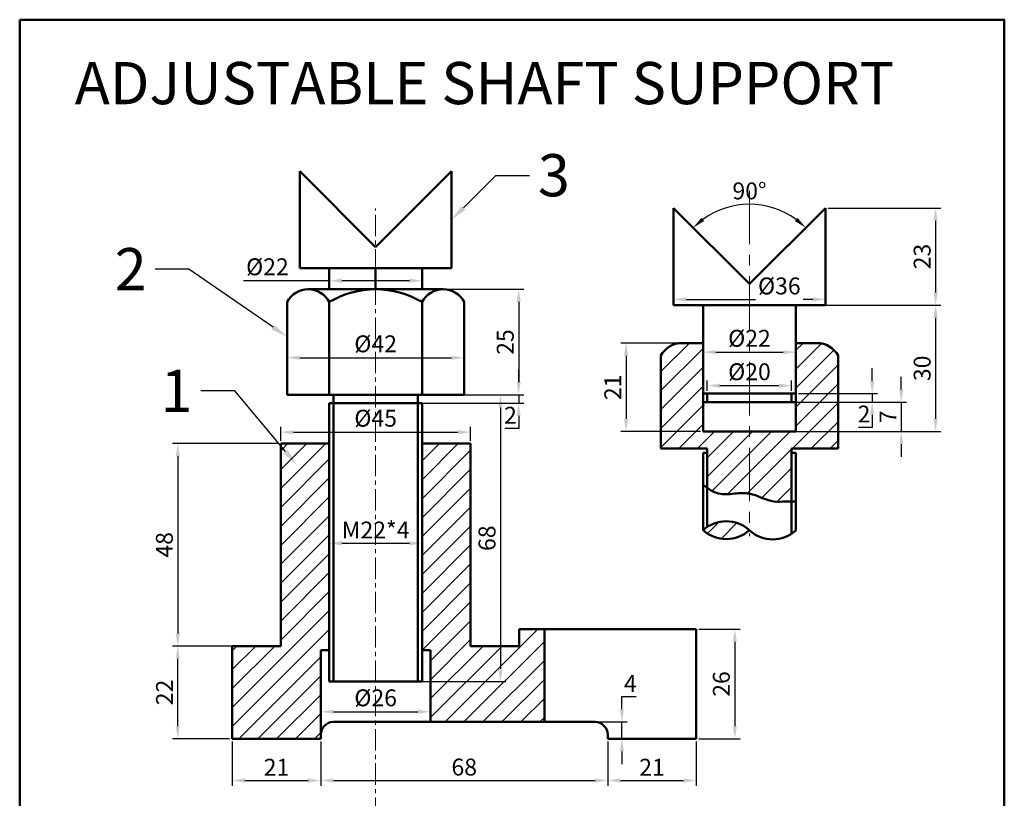
# Model space of a CAD drawing. Units: millimetres. Extents: x 458 to 691, y 231 to 528.
# Tile 2 of 2: x 458 to 691, y 343 to 528. Entities that reach past the tile are written whole.
import ezdxf
from ezdxf import colors
from ezdxf.entities.mleader import LeaderData, LeaderLine
from ezdxf.math import Vec2, Vec3

# ---------------------------------------------------------------- set-up
doc = ezdxf.new("R2010")
doc.units = ezdxf.units.MM
doc.header["$LTSCALE"] = 0.4
doc.linetypes.add('CENTER', pattern=[50.8, 31.75, -6.35, 6.35, -6.35])
for name, color, linetype, lineweight in [('M-CNTR', 1, 'CENTER', 18), ('M-DIMS', 2, 'Continuous', 25), ('M-HATC', 8, 'Continuous', 18), ('M-OUTL', 7, 'Continuous', 50), ('M-TEXT', 3, 'Continuous', 25)]:
    doc.layers.add(name, color=color, linetype=linetype, lineweight=lineweight)
doc.styles.get("Standard").update_dxf_attribs({"font": 'arial.ttf'})
doc.dimstyles.new('ISO-25', dxfattribs={"dimtxt": 4, "dimasz": 3, "dimexe": 1.25, "dimexo": 0.625, "dimtad": 1, "dimtoh": 1, "dimtxsty": 'Standard', "dimcen": 2.5, "dimadec": 0, "dimazin": 0, "dimtfac": 1, "dimtmove": 0, "dimatfit": 3, "dimfxl": 1, "dimarcsym": 0})

# ---------------------------------------------------------------- blocks, each defined once
blk = doc.blocks.new('*D1')
at = {"layer": 'Defpoints', "color": 0, "ltscale": 0.4, "transparency": 16777216}
for p in [(635.76, 483.24), (612.87, 483), (648.87, 483), (630.87, 465), (630.87, 465)]:
    blk.add_point(p, dxfattribs=at)
at = {"layer": 'M-DIMS', "color": 0, "lineweight": -2, "ltscale": 0.4, "transparency": 16777216}
blk.add_arc((630.87, 465), 18.88, 54.1129, 125.8871, dxfattribs=at)
at = {"layer": 'M-DIMS', "color": 0, "ltscale": 0.4, "transparency": 16777216}
for points in [[(620.13, 479.92), (619.48, 480.68), (617.52, 478.35)], [(642.26, 480.68), (641.61, 479.92), (644.22, 478.35)]]:
    blk.add_solid(points, dxfattribs=at)
at = {"layer": 'M-DIMS', "color": 0, "ltscale": 0.4, "transparency": 16777216, "insert": (630.87, 486.55), "char_height": 4, "attachment_point": 5}
blk.add_mtext('90°', dxfattribs=at)
blk = doc.blocks.new('*D2')
at = {"layer": 'Defpoints', "color": 0, "ltscale": 0.4, "transparency": 16777216}
for p in [(612.87, 460), (648.87, 461.34), (648.87, 460)]:
    blk.add_point(p, dxfattribs=at)
at = {"layer": 'M-DIMS', "color": 0, "lineweight": -2, "ltscale": 0.4, "transparency": 16777216}
for p, q in [((612.87, 460.63), (612.87, 462.59)), ((648.87, 460.63), (648.87, 462.59)), ((615.87, 461.34), (632.29, 461.34)), ((645.87, 461.34), (643.62, 461.34))]:
    blk.add_line(p, q, dxfattribs=at)
at = {"layer": 'M-DIMS', "color": 0, "ltscale": 0.4, "transparency": 16777216}
for points in [[(615.87, 461.84), (615.87, 460.84), (612.87, 461.34)], [(645.87, 461.84), (645.87, 460.84), (648.87, 461.34)]]:
    blk.add_solid(points, dxfattribs=at)
at = {"layer": 'M-DIMS', "color": 0, "ltscale": 0.4, "transparency": 16777216, "insert": (637.95, 464.01), "char_height": 4, "attachment_point": 5}
blk.add_mtext('%%C36', dxfattribs=at)
blk = doc.blocks.new('*D3')
at = {"layer": 'Defpoints', "color": 0, "ltscale": 0.4, "transparency": 16777216}
for p in [(641.87, 448.83), (619.87, 446.06), (641.87, 446.06)]:
    blk.add_point(p, dxfattribs=at)
at = {"layer": 'M-DIMS', "color": 0, "lineweight": -2, "ltscale": 0.4, "transparency": 16777216}
for p, q in [((619.87, 446.68), (619.87, 450.08)), ((622.87, 448.83), (638.87, 448.83)), ((641.87, 446.68), (641.87, 450.08))]:
    blk.add_line(p, q, dxfattribs=at)
at = {"layer": 'M-DIMS', "color": 0, "ltscale": 0.4, "transparency": 16777216}
for points in [[(622.87, 449.33), (622.87, 448.33), (619.87, 448.83)], [(638.87, 449.33), (638.87, 448.33), (641.87, 448.83)]]:
    blk.add_solid(points, dxfattribs=at)
at = {"layer": 'M-DIMS', "color": 0, "ltscale": 0.4, "transparency": 16777216, "insert": (630.87, 451.61), "char_height": 4, "attachment_point": 5}
blk.add_mtext('%%C22', dxfattribs=at)
blk = doc.blocks.new('*D4')
at = {"layer": 'Defpoints', "color": 0, "ltscale": 0.4, "transparency": 16777216}
for p in [(620.87, 439), (640.87, 440.89), (640.87, 439)]:
    blk.add_point(p, dxfattribs=at)
at = {"layer": 'M-DIMS', "color": 0, "lineweight": -2, "ltscale": 0.4, "transparency": 16777216}
for p, q in [((620.87, 439.63), (620.87, 442.14)), ((640.87, 439.63), (640.87, 442.14)), ((623.87, 440.89), (637.87, 440.89))]:
    blk.add_line(p, q, dxfattribs=at)
at = {"layer": 'M-DIMS', "color": 0, "ltscale": 0.4, "transparency": 16777216}
for points in [[(623.87, 441.39), (623.87, 440.39), (620.87, 440.89)], [(637.87, 441.39), (637.87, 440.39), (640.87, 440.89)]]:
    blk.add_solid(points, dxfattribs=at)
at = {"layer": 'M-DIMS', "color": 0, "ltscale": 0.4, "transparency": 16777216, "insert": (630.87, 443.67), "char_height": 4, "attachment_point": 5}
blk.add_mtext('%%C20', dxfattribs=at)
blk = doc.blocks.new('*D5')
at = {"layer": 'Defpoints', "color": 0, "ltscale": 0.4, "transparency": 16777216}
for p in [(617.37, 451), (601.63, 430), (619.87, 430)]:
    blk.add_point(p, dxfattribs=at)
at = {"layer": 'M-DIMS', "color": 0, "lineweight": -2, "ltscale": 0.4, "transparency": 16777216}
for p, q in [((616.75, 451), (600.38, 451)), ((601.63, 448), (601.63, 433)), ((619.25, 430), (600.38, 430))]:
    blk.add_line(p, q, dxfattribs=at)
at = {"layer": 'M-DIMS', "color": 0, "ltscale": 0.4, "transparency": 16777216}
for points in [[(601.13, 448), (602.13, 448), (601.63, 451)], [(601.13, 433), (602.13, 433), (601.63, 430)]]:
    blk.add_solid(points, dxfattribs=at)
at = {"layer": 'M-DIMS', "color": 0, "ltscale": 0.4, "transparency": 16777216, "insert": (599, 440.5), "char_height": 4, "attachment_point": 5, "rotation": 90}
blk.add_mtext('21', dxfattribs=at)
blk = doc.blocks.new('*D6')
at = {"layer": 'Defpoints', "color": 0, "ltscale": 0.4, "transparency": 16777216}
for p in [(641.87, 439), (641.87, 437), (659.97, 437)]:
    blk.add_point(p, dxfattribs=at)
at = {"layer": 'M-DIMS', "color": 0, "lineweight": -2, "ltscale": 0.4, "transparency": 16777216}
for p, q in [((659.97, 442), (659.97, 445)), ((642.5, 439), (661.22, 439)), ((659.97, 439), (659.97, 437)), ((642.5, 437), (661.22, 437)), ((659.97, 434), (659.97, 431)), ((659.97, 431), (656.7, 431))]:
    blk.add_line(p, q, dxfattribs=at)
at = {"layer": 'M-DIMS', "color": 0, "ltscale": 0.4, "transparency": 16777216}
for points in [[(659.47, 442), (660.47, 442), (659.97, 439)], [(659.47, 434), (660.47, 434), (659.97, 437)]]:
    blk.add_solid(points, dxfattribs=at)
at = {"layer": 'M-DIMS', "color": 0, "ltscale": 0.4, "transparency": 16777216, "insert": (658.02, 433.64), "char_height": 4, "attachment_point": 5}
blk.add_mtext('2', dxfattribs=at)
blk = doc.blocks.new('*D7')
at = {"layer": 'Defpoints', "color": 0, "ltscale": 0.4, "transparency": 16777216}
for p in [(639.64, 437), (639.64, 430), (666.85, 430)]:
    blk.add_point(p, dxfattribs=at)
at = {"layer": 'M-DIMS', "color": 0, "lineweight": -2, "ltscale": 0.4, "transparency": 16777216}
for p, q in [((666.85, 440), (666.85, 443)), ((640.27, 437), (668.1, 437)), ((666.85, 437), (666.85, 430)), ((640.27, 430), (668.1, 430)), ((666.85, 427), (666.85, 424))]:
    blk.add_line(p, q, dxfattribs=at)
at = {"layer": 'M-DIMS', "color": 0, "ltscale": 0.4, "transparency": 16777216}
for points in [[(666.35, 440), (667.35, 440), (666.85, 437)], [(666.35, 427), (667.35, 427), (666.85, 430)]]:
    blk.add_solid(points, dxfattribs=at)
at = {"layer": 'M-DIMS', "color": 0, "ltscale": 0.4, "transparency": 16777216, "insert": (664.23, 433.5), "char_height": 4, "attachment_point": 5, "rotation": 90}
blk.add_mtext('7', dxfattribs=at)
blk = doc.blocks.new('*D8')
at = {"layer": 'Defpoints', "color": 0, "ltscale": 0.4, "transparency": 16777216}
for p in [(641.87, 460), (641.87, 430), (674.99, 430)]:
    blk.add_point(p, dxfattribs=at)
at = {"layer": 'M-DIMS', "color": 0, "lineweight": -2, "ltscale": 0.4, "transparency": 16777216}
for p, q in [((642.5, 460), (676.24, 460)), ((674.99, 457), (674.99, 433)), ((642.5, 430), (676.24, 430))]:
    blk.add_line(p, q, dxfattribs=at)
at = {"layer": 'M-DIMS', "color": 0, "ltscale": 0.4, "transparency": 16777216}
for points in [[(674.49, 457), (675.49, 457), (674.99, 460)], [(674.49, 433), (675.49, 433), (674.99, 430)]]:
    blk.add_solid(points, dxfattribs=at)
at = {"layer": 'M-DIMS', "color": 0, "ltscale": 0.4, "transparency": 16777216, "insert": (672.32, 445), "char_height": 4, "attachment_point": 5, "rotation": 90}
blk.add_mtext('30', dxfattribs=at)
blk = doc.blocks.new('*D9')
at = {"layer": 'Defpoints', "color": 0, "ltscale": 0.4, "transparency": 16777216}
for p in [(648.87, 483), (648.87, 460), (674.99, 460)]:
    blk.add_point(p, dxfattribs=at)
at = {"layer": 'M-DIMS', "color": 0, "lineweight": -2, "ltscale": 0.4, "transparency": 16777216}
for p, q in [((649.5, 483), (676.24, 483)), ((674.99, 480), (674.99, 463)), ((649.5, 460), (676.24, 460))]:
    blk.add_line(p, q, dxfattribs=at)
at = {"layer": 'M-DIMS', "color": 0, "ltscale": 0.4, "transparency": 16777216}
for points in [[(674.49, 480), (675.49, 480), (674.99, 483)], [(674.49, 463), (675.49, 463), (674.99, 460)]]:
    blk.add_solid(points, dxfattribs=at)
at = {"layer": 'M-DIMS', "color": 0, "ltscale": 0.4, "transparency": 16777216, "insert": (672.32, 471.5), "char_height": 4, "attachment_point": 5, "rotation": 90}
blk.add_mtext('23', dxfattribs=at)
blk = doc.blocks.new('*D10')
at = {"layer": 'Defpoints', "color": 0, "ltscale": 0.4, "transparency": 16777216}
for p in [(531.27, 467.48), (553.27, 466.23), (553.27, 465.77)]:
    blk.add_point(p, dxfattribs=at)
at = {"layer": 'M-DIMS', "color": 0, "lineweight": -2, "ltscale": 0.4, "transparency": 16777216}
for p, q in [((531.27, 466.86), (531.27, 464.52)), ((531.27, 465.77), (510.97, 465.77)), ((550.27, 465.77), (534.27, 465.77)), ((553.27, 465.61), (553.27, 464.52))]:
    blk.add_line(p, q, dxfattribs=at)
at = {"layer": 'M-DIMS', "color": 0, "ltscale": 0.4, "transparency": 16777216}
for points in [[(534.27, 466.27), (534.27, 465.27), (531.27, 465.77)], [(550.27, 466.27), (550.27, 465.27), (553.27, 465.77)]]:
    blk.add_solid(points, dxfattribs=at)
at = {"layer": 'M-DIMS', "color": 0, "ltscale": 0.4, "transparency": 16777216, "insert": (516.62, 468.55), "char_height": 4, "attachment_point": 5}
blk.add_mtext('%%C22', dxfattribs=at)
blk = doc.blocks.new('*D11')
at = {"layer": 'Defpoints', "color": 0, "ltscale": 0.4, "transparency": 16777216}
for p in [(521.27, 449.73), (563.27, 449.73), (563.27, 447.51)]:
    blk.add_point(p, dxfattribs=at)
at = {"layer": 'M-DIMS', "color": 0, "lineweight": -2, "ltscale": 0.4, "transparency": 16777216}
for p, q in [((521.27, 449.11), (521.27, 446.26)), ((563.27, 449.11), (563.27, 446.26)), ((524.27, 447.51), (560.27, 447.51))]:
    blk.add_line(p, q, dxfattribs=at)
at = {"layer": 'M-DIMS', "color": 0, "ltscale": 0.4, "transparency": 16777216}
for points in [[(524.27, 448.01), (524.27, 447.01), (521.27, 447.51)], [(560.27, 448.01), (560.27, 447.01), (563.27, 447.51)]]:
    blk.add_solid(points, dxfattribs=at)
at = {"layer": 'M-DIMS', "color": 0, "ltscale": 0.4, "transparency": 16777216, "insert": (542.27, 450.29), "char_height": 4, "attachment_point": 5}
blk.add_mtext('%%C42', dxfattribs=at)
blk = doc.blocks.new('*D12')
at = {"layer": 'Defpoints', "color": 0, "ltscale": 0.4, "transparency": 16777216}
for p in [(558.27, 463.73), (558.27, 438.73), (576.17, 438.73)]:
    blk.add_point(p, dxfattribs=at)
at = {"layer": 'M-DIMS', "color": 0, "lineweight": -2, "ltscale": 0.4, "transparency": 16777216}
for p, q in [((558.9, 463.73), (577.42, 463.73)), ((576.17, 460.73), (576.17, 441.73)), ((558.9, 438.73), (577.42, 438.73))]:
    blk.add_line(p, q, dxfattribs=at)
at = {"layer": 'M-DIMS', "color": 0, "ltscale": 0.4, "transparency": 16777216}
for points in [[(575.67, 460.73), (576.67, 460.73), (576.17, 463.73)], [(575.67, 441.73), (576.67, 441.73), (576.17, 438.73)]]:
    blk.add_solid(points, dxfattribs=at)
at = {"layer": 'M-DIMS', "color": 0, "ltscale": 0.4, "transparency": 16777216, "insert": (573.51, 451.23), "char_height": 4, "attachment_point": 5, "rotation": 90}
blk.add_mtext('25', dxfattribs=at)
blk = doc.blocks.new('*D13')
at = {"layer": 'Defpoints', "color": 0, "ltscale": 0.4, "transparency": 16777216}
for p in [(552.27, 438.73), (552.27, 436.73), (576.17, 436.73)]:
    blk.add_point(p, dxfattribs=at)
at = {"layer": 'M-DIMS', "color": 0, "lineweight": -2, "ltscale": 0.4, "transparency": 16777216}
for p, q in [((576.17, 441.73), (576.17, 444.73)), ((552.9, 438.73), (577.42, 438.73)), ((576.17, 438.73), (576.17, 436.73)), ((552.9, 436.73), (577.42, 436.73)), ((576.17, 433.73), (576.17, 430.73)), ((576.17, 430.73), (572.9, 430.73))]:
    blk.add_line(p, q, dxfattribs=at)
at = {"layer": 'M-DIMS', "color": 0, "ltscale": 0.4, "transparency": 16777216}
for points in [[(575.67, 441.73), (576.67, 441.73), (576.17, 438.73)], [(575.67, 433.73), (576.67, 433.73), (576.17, 436.73)]]:
    blk.add_solid(points, dxfattribs=at)
at = {"layer": 'M-DIMS', "color": 0, "ltscale": 0.4, "transparency": 16777216, "insert": (574.22, 433.36), "char_height": 4, "attachment_point": 5}
blk.add_mtext('2', dxfattribs=at)
blk = doc.blocks.new('*D14')
at = {"layer": 'Defpoints', "color": 0, "ltscale": 0.4, "transparency": 16777216}
for p in [(564.77, 429.87), (519.77, 427.16), (564.77, 427.16)]:
    blk.add_point(p, dxfattribs=at)
at = {"layer": 'M-DIMS', "color": 0, "lineweight": -2, "ltscale": 0.4, "transparency": 16777216}
for p, q in [((519.77, 427.78), (519.77, 431.12)), ((522.77, 429.87), (561.77, 429.87)), ((564.77, 427.78), (564.77, 431.12))]:
    blk.add_line(p, q, dxfattribs=at)
at = {"layer": 'M-DIMS', "color": 0, "ltscale": 0.4, "transparency": 16777216}
for points in [[(522.77, 430.37), (522.77, 429.37), (519.77, 429.87)], [(561.77, 430.37), (561.77, 429.37), (564.77, 429.87)]]:
    blk.add_solid(points, dxfattribs=at)
at = {"layer": 'M-DIMS', "color": 0, "ltscale": 0.4, "transparency": 16777216, "insert": (542.27, 432.65), "char_height": 4, "attachment_point": 5}
blk.add_mtext('%%C45', dxfattribs=at)
blk = doc.blocks.new('*D15')
at = {"layer": 'Defpoints', "color": 0, "ltscale": 0.4, "transparency": 16777216}
for p in [(569.66, 438.73), (542.27, 370.73), (571.85, 370.73)]:
    blk.add_point(p, dxfattribs=at)
at = {"layer": 'M-DIMS', "color": 0, "lineweight": -2, "ltscale": 0.4, "transparency": 16777216}
for p, q in [((570.28, 438.73), (573.1, 438.73)), ((571.85, 435.73), (571.85, 373.73)), ((542.9, 370.73), (573.1, 370.73))]:
    blk.add_line(p, q, dxfattribs=at)
at = {"layer": 'M-DIMS', "color": 0, "ltscale": 0.4, "transparency": 16777216}
for points in [[(571.35, 435.73), (572.35, 435.73), (571.85, 438.73)], [(571.35, 373.73), (572.35, 373.73), (571.85, 370.73)]]:
    blk.add_solid(points, dxfattribs=at)
at = {"layer": 'M-DIMS', "color": 0, "ltscale": 0.4, "transparency": 16777216, "insert": (569.19, 404.73), "char_height": 4, "attachment_point": 5, "rotation": 90}
blk.add_mtext('68', dxfattribs=at)
blk = doc.blocks.new('*D16')
at = {"layer": 'Defpoints', "color": 0, "ltscale": 0.4, "transparency": 16777216}
for p in [(531.27, 403.73), (553.27, 403.73), (553.27, 403.52)]:
    blk.add_point(p, dxfattribs=at)
at = {"layer": 'M-DIMS', "color": 0, "lineweight": -2, "ltscale": 0.4, "transparency": 16777216}
for p, q in [((531.27, 403.11), (531.27, 402.27)), ((534.27, 403.52), (550.27, 403.52)), ((553.27, 403.11), (553.27, 402.27))]:
    blk.add_line(p, q, dxfattribs=at)
at = {"layer": 'M-DIMS', "color": 0, "ltscale": 0.4, "transparency": 16777216}
for points in [[(534.27, 404.02), (534.27, 403.02), (531.27, 403.52)], [(550.27, 404.02), (550.27, 403.02), (553.27, 403.52)]]:
    blk.add_solid(points, dxfattribs=at)
at = {"layer": 'M-DIMS', "color": 0, "ltscale": 0.4, "transparency": 16777216, "insert": (542.27, 406.15), "char_height": 4, "attachment_point": 5}
blk.add_mtext('M22*4', dxfattribs=at)
blk = doc.blocks.new('*D17')
at = {"layer": 'Defpoints', "color": 0, "ltscale": 0.4, "transparency": 16777216}
for p in [(529.27, 364.88), (555.27, 364.88), (555.27, 363.58)]:
    blk.add_point(p, dxfattribs=at)
at = {"layer": 'M-DIMS', "color": 0, "lineweight": -2, "ltscale": 0.4, "transparency": 16777216}
for p, q in [((529.27, 364.26), (529.27, 362.33)), ((555.27, 364.26), (555.27, 362.33)), ((532.27, 363.58), (552.27, 363.58))]:
    blk.add_line(p, q, dxfattribs=at)
at = {"layer": 'M-DIMS', "color": 0, "ltscale": 0.4, "transparency": 16777216}
for points in [[(532.27, 364.08), (532.27, 363.08), (529.27, 363.58)], [(552.27, 364.08), (552.27, 363.08), (555.27, 363.58)]]:
    blk.add_solid(points, dxfattribs=at)
at = {"layer": 'M-DIMS', "color": 0, "ltscale": 0.4, "transparency": 16777216, "insert": (542.27, 366.36), "char_height": 4, "attachment_point": 5}
blk.add_mtext('%%C26', dxfattribs=at)
blk = doc.blocks.new('*D18')
at = {"layer": 'Defpoints', "color": 0, "ltscale": 0.4, "transparency": 16777216}
for p in [(519.77, 427.16), (495.38, 379.16), (519.77, 379.16)]:
    blk.add_point(p, dxfattribs=at)
at = {"layer": 'M-DIMS', "color": 0, "lineweight": -2, "ltscale": 0.4, "transparency": 16777216}
for p, q in [((519.15, 427.16), (494.13, 427.16)), ((495.38, 424.16), (495.38, 382.16)), ((519.15, 379.16), (494.13, 379.16))]:
    blk.add_line(p, q, dxfattribs=at)
at = {"layer": 'M-DIMS', "color": 0, "ltscale": 0.4, "transparency": 16777216}
for points in [[(494.88, 424.16), (495.88, 424.16), (495.38, 427.16)], [(494.88, 382.16), (495.88, 382.16), (495.38, 379.16)]]:
    blk.add_solid(points, dxfattribs=at)
at = {"layer": 'M-DIMS', "color": 0, "ltscale": 0.4, "transparency": 16777216, "insert": (492.72, 403.16), "char_height": 4, "attachment_point": 5, "rotation": 90}
blk.add_mtext('48', dxfattribs=at)
blk = doc.blocks.new('*D19')
at = {"layer": 'Defpoints', "color": 0, "ltscale": 0.4, "transparency": 16777216}
for p in [(495.38, 379.16), (508.27, 379.16), (508.27, 357.16)]:
    blk.add_point(p, dxfattribs=at)
at = {"layer": 'M-DIMS', "color": 0, "lineweight": -2, "ltscale": 0.4, "transparency": 16777216}
for p, q in [((507.65, 379.16), (494.13, 379.16)), ((495.38, 360.16), (495.38, 376.16)), ((507.65, 357.16), (494.13, 357.16))]:
    blk.add_line(p, q, dxfattribs=at)
at = {"layer": 'M-DIMS', "color": 0, "ltscale": 0.4, "transparency": 16777216}
for points in [[(494.88, 376.16), (495.88, 376.16), (495.38, 379.16)], [(494.88, 360.16), (495.88, 360.16), (495.38, 357.16)]]:
    blk.add_solid(points, dxfattribs=at)
at = {"layer": 'M-DIMS', "color": 0, "ltscale": 0.4, "transparency": 16777216, "insert": (492.75, 368.16), "char_height": 4, "attachment_point": 5, "rotation": 90}
blk.add_mtext('22', dxfattribs=at)
blk = doc.blocks.new('*D20')
at = {"layer": 'Defpoints', "color": 0, "ltscale": 0.4, "transparency": 16777216}
for p in [(508.27, 357.16), (529.27, 357.16), (529.27, 347.28)]:
    blk.add_point(p, dxfattribs=at)
at = {"layer": 'M-DIMS', "color": 0, "lineweight": -2, "ltscale": 0.4, "transparency": 16777216}
for p, q in [((508.27, 356.53), (508.27, 346.03)), ((529.27, 356.53), (529.27, 346.03)), ((511.27, 347.28), (526.27, 347.28))]:
    blk.add_line(p, q, dxfattribs=at)
at = {"layer": 'M-DIMS', "color": 0, "ltscale": 0.4, "transparency": 16777216}
for points in [[(511.27, 347.78), (511.27, 346.78), (508.27, 347.28)], [(526.27, 347.78), (526.27, 346.78), (529.27, 347.28)]]:
    blk.add_solid(points, dxfattribs=at)
at = {"layer": 'M-DIMS', "color": 0, "ltscale": 0.4, "transparency": 16777216, "insert": (518.77, 349.91), "char_height": 4, "attachment_point": 5}
blk.add_mtext('21', dxfattribs=at)
blk = doc.blocks.new('*D21')
at = {"layer": 'Defpoints', "color": 0, "ltscale": 0.4, "transparency": 16777216}
for p in [(529.27, 357.16), (597.27, 357.16), (597.27, 347.28)]:
    blk.add_point(p, dxfattribs=at)
at = {"layer": 'M-DIMS', "color": 0, "lineweight": -2, "ltscale": 0.4, "transparency": 16777216}
for p, q in [((529.27, 356.53), (529.27, 346.03)), ((597.27, 356.53), (597.27, 346.03)), ((532.27, 347.28), (594.27, 347.28))]:
    blk.add_line(p, q, dxfattribs=at)
at = {"layer": 'M-DIMS', "color": 0, "ltscale": 0.4, "transparency": 16777216}
for points in [[(532.27, 347.78), (532.27, 346.78), (529.27, 347.28)], [(594.27, 347.78), (594.27, 346.78), (597.27, 347.28)]]:
    blk.add_solid(points, dxfattribs=at)
at = {"layer": 'M-DIMS', "color": 0, "ltscale": 0.4, "transparency": 16777216, "insert": (563.27, 349.95), "char_height": 4, "attachment_point": 5}
blk.add_mtext('68', dxfattribs=at)
blk = doc.blocks.new('*D22')
at = {"layer": 'Defpoints', "color": 0, "ltscale": 0.4, "transparency": 16777216}
for p in [(591.35, 361.16), (600.64, 361.16), (601.78, 357.16)]:
    blk.add_point(p, dxfattribs=at)
at = {"layer": 'M-DIMS', "color": 0, "lineweight": -2, "ltscale": 0.4, "transparency": 16777216}
for p, q in [((600.64, 364.16), (600.64, 367.16)), ((600.64, 367.16), (604.03, 367.16)), ((591.98, 361.16), (601.89, 361.16)), ((600.64, 357.16), (600.64, 361.16)), ((601.15, 357.16), (599.39, 357.16)), ((600.64, 354.16), (600.64, 351.16))]:
    blk.add_line(p, q, dxfattribs=at)
at = {"layer": 'M-DIMS', "color": 0, "ltscale": 0.4, "transparency": 16777216}
for points in [[(600.14, 364.16), (601.14, 364.16), (600.64, 361.16)], [(600.14, 354.16), (601.14, 354.16), (600.64, 357.16)]]:
    blk.add_solid(points, dxfattribs=at)
at = {"layer": 'M-DIMS', "color": 0, "ltscale": 0.4, "transparency": 16777216, "insert": (602.65, 369.78), "char_height": 4, "attachment_point": 5}
blk.add_mtext('4', dxfattribs=at)
blk = doc.blocks.new('*D23')
at = {"layer": 'Defpoints', "color": 0, "ltscale": 0.4, "transparency": 16777216}
for p in [(597.27, 357.16), (618.27, 357.16), (618.27, 347.28)]:
    blk.add_point(p, dxfattribs=at)
at = {"layer": 'M-DIMS', "color": 0, "lineweight": -2, "ltscale": 0.4, "transparency": 16777216}
for p, q in [((597.27, 356.53), (597.27, 346.03)), ((618.27, 356.53), (618.27, 346.03)), ((600.27, 347.28), (615.27, 347.28))]:
    blk.add_line(p, q, dxfattribs=at)
at = {"layer": 'M-DIMS', "color": 0, "ltscale": 0.4, "transparency": 16777216}
for points in [[(600.27, 347.78), (600.27, 346.78), (597.27, 347.28)], [(615.27, 347.78), (615.27, 346.78), (618.27, 347.28)]]:
    blk.add_solid(points, dxfattribs=at)
at = {"layer": 'M-DIMS', "color": 0, "ltscale": 0.4, "transparency": 16777216, "insert": (607.77, 349.91), "char_height": 4, "attachment_point": 5}
blk.add_mtext('21', dxfattribs=at)
blk = doc.blocks.new('*D24')
at = {"layer": 'Defpoints', "color": 0, "ltscale": 0.4, "transparency": 16777216}
for p in [(618.27, 383.16), (618.27, 357.16), (627.4, 357.16)]:
    blk.add_point(p, dxfattribs=at)
at = {"layer": 'M-DIMS', "color": 0, "lineweight": -2, "ltscale": 0.4, "transparency": 16777216}
for p, q in [((618.9, 383.16), (628.65, 383.16)), ((627.4, 380.16), (627.4, 360.16)), ((618.9, 357.16), (628.65, 357.16))]:
    blk.add_line(p, q, dxfattribs=at)
at = {"layer": 'M-DIMS', "color": 0, "ltscale": 0.4, "transparency": 16777216}
for points in [[(626.9, 380.16), (627.9, 380.16), (627.4, 383.16)], [(626.9, 360.16), (627.9, 360.16), (627.4, 357.16)]]:
    blk.add_solid(points, dxfattribs=at)
at = {"layer": 'M-DIMS', "color": 0, "ltscale": 0.4, "transparency": 16777216, "insert": (624.73, 370.16), "char_height": 4, "attachment_point": 5, "rotation": 90}
blk.add_mtext('26', dxfattribs=at)

msp = doc.modelspace()

# ---------------------------------------------------------------- hatches: boundary and pattern name
at = {"layer": 'M-HATC', "ltscale": 0.4}
h = msp.add_hatch(dxfattribs=at)
h.set_pattern_fill('ANSI31', color=256)
h.set_pattern_definition([(45, (-8.7276, -12.7276), (-2.245064, 2.245064), [])])
edge = h.paths.add_edge_path()
edge.add_line((619.871, 448.002), (619.871, 451.002))
edge.add_line((619.871, 451.002), (614.871, 451.002))
edge.add_arc((614.871, 445.336), 5.667, 90, 151.92751)
edge.add_line((609.871, 448.002), (609.871, 426.002))
edge.add_line((609.871, 426.002), (619.871, 426.002))
edge.add_line((619.871, 426.002), (620.871, 426.002))
edge.add_line((620.871, 426.002), (620.871, 425.002))
edge.add_line((620.871, 425.002), (620.871, 416.66))
edge.add_spline(control_points=[(620.871, 416.66), (621.726, 416.055), (623.692, 414.881), (627.273, 415.321), (629.73, 415.508), (630.871, 415.299)], knot_values=[1.1963564, 1.1963564, 1.1963564, 1.1963564, 4.2434705, 8.0269006, 11.5560134, 11.5560134, 11.5560134, 11.5560134], degree=3, periodic=0)
edge.add_line((630.871, 415.299), (630.871, 430.002))
edge.add_line((630.871, 430.002), (619.871, 430.002))
edge.add_line((619.871, 430.002), (619.871, 448.002))
edge = h.paths.add_edge_path()
edge.add_arc((646.871, 445.336), 5.667, 28.07249, 90)
edge.add_line((646.871, 451.002), (641.871, 451.002))
edge.add_line((641.871, 451.002), (641.871, 430.002))
edge.add_line((641.871, 430.002), (630.871, 430.002))
edge.add_line((630.871, 430.002), (630.871, 415.299))
edge.add_spline(control_points=[(630.871, 415.299), (632.83, 414.94), (635.517, 413.113), (638.999, 413.444), (640.411, 413.45), (640.871, 413.447)], knot_values=[11.5560134, 11.5560134, 11.5560134, 11.5560134, 17.6166042, 20.465853, 21.8484092, 21.8484092, 21.8484092, 21.8484092], degree=3, periodic=0)
edge.add_line((640.871, 413.447), (640.871, 425.002))
edge.add_line((640.871, 425.002), (640.871, 426.002))
edge.add_line((640.871, 426.002), (641.871, 426.002))
edge.add_line((641.871, 426.002), (651.871, 426.002))
edge.add_line((651.871, 426.002), (651.871, 448.002))
h.paths.add_polyline_path([(619.871, 406.629, 0.3827344), (630.871, 406.629, 0.3827344)])
h = msp.add_hatch(dxfattribs=at)
h.set_pattern_fill('ANSI31', color=256)
h.paths.add_polyline_path([(529.271, 378.156), (531.271, 378.156), (531.271, 427.156), (519.771, 427.156), (519.771, 379.156), (508.271, 379.156), (508.271, 357.156), (529.271, 357.156)])
h.paths.add_polyline_path([(582.271, 383.156), (576.271, 383.156), (576.271, 379.156), (564.771, 379.156), (564.771, 427.156), (553.271, 427.156), (553.271, 378.156), (555.271, 378.156), (555.271, 361.156), (582.271, 361.156)])

# ---------------------------------------------------------------- linework, layer by layer
at = {"layer": 'M-CNTR'}
msp.add_line((630.871, 487.143), (630.871, 405.224), dxfattribs=at)
at = {"layer": 'M-CNTR', "ltscale": 0.4}
msp.add_line((542.271, 248.744), (542.271, 482.881), dxfattribs=at)
at = {"layer": 'M-OUTL'}
for p, q in [((524.271, 468.73), (524.271, 491.73)), ((524.271, 491.73), (542.271, 473.73)), ((560.271, 491.73), (542.271, 473.73)), ((560.271, 468.73), (560.271, 491.73)), ((612.871, 460.002), (612.871, 483.002)), ((612.871, 483.002), (630.871, 465.002)), ((648.871, 483.002), (630.871, 465.002)), ((648.871, 460.002), (648.871, 483.002)), ((524.271, 468.73), (560.271, 468.73)), ((531.271, 468.73), (531.271, 463.73)), ((542.271, 468.73), (542.271, 463.73)), ((553.271, 463.73), (553.271, 468.73)), ((558.271, 463.73), (526.271, 463.73)), ((521.271, 460.73), (521.271, 438.73)), ((531.271, 460.73), (531.271, 438.73)), ((531.271, 460.73), (531.271, 438.73)), ((553.271, 460.73), (553.271, 438.73)), ((553.271, 438.73), (553.271, 460.73)), ((563.271, 438.73), (563.271, 460.73)), ((612.871, 460.002), (648.871, 460.002)), ((619.871, 460.002), (619.871, 434.002)), ((641.871, 434.002), (641.871, 460.002)), ((619.871, 451.002), (614.871, 451.002)), ((646.871, 451.002), (641.871, 451.002)), ((609.871, 448.002), (609.871, 426.002)), ((619.871, 448.002), (619.871, 430.002)), ((641.871, 448.002), (641.871, 430.002)), ((651.871, 426.002), (651.871, 448.002)), ((521.271, 438.73), (563.271, 438.73)), ((531.271, 438.73), (553.271, 438.73)), ((619.871, 437.002), (619.871, 439.002)), ((619.871, 439.002), (641.871, 439.002)), ((620.871, 439.002), (620.871, 437.002)), ((640.871, 439.002), (640.871, 437.002)), ((641.871, 437.002), (619.871, 437.002)), ((619.871, 430.002), (641.871, 430.002)), ((609.871, 426.002), (619.871, 426.002)), ((619.871, 426.002), (620.871, 426.002)), ((619.871, 425.002), (619.871, 406.629)), ((620.871, 425.002), (619.871, 425.002)), ((620.871, 426.002), (620.871, 425.002)), ((641.871, 426.002), (640.871, 426.002)), ((640.871, 426.002), (640.871, 425.002)), ((640.871, 425.002), (641.871, 425.002)), ((641.871, 426.002), (651.871, 426.002)), ((641.871, 425.002), (641.871, 406.545))]:
    msp.add_line(p, q, dxfattribs=at)
at = {"layer": 'M-OUTL', "ltscale": 0.4}
for p, q in [((532.271, 438.73), (532.271, 436.73)), ((532.271, 438.73), (532.271, 370.73)), ((552.271, 438.73), (552.271, 436.73)), ((552.271, 370.73), (552.271, 438.73)), ((531.271, 436.73), (531.271, 370.73)), ((553.271, 436.73), (531.271, 436.73)), ((553.271, 370.73), (553.271, 436.73)), ((531.271, 427.156), (519.771, 427.156)), ((519.771, 427.156), (519.771, 379.156)), ((553.271, 427.156), (564.771, 427.156)), ((564.771, 427.156), (564.771, 379.156)), ((620.871, 425.002), (620.871, 407.396)), ((640.871, 425.002), (640.871, 405.778)), ((618.271, 383.156), (576.271, 383.156)), ((576.271, 379.156), (576.271, 383.156)), ((582.271, 361.156), (582.271, 383.156)), ((618.271, 357.156), (618.271, 383.156)), ((508.271, 357.156), (508.271, 379.156)), ((508.271, 379.156), (519.771, 379.156)), ((531.271, 378.156), (529.271, 378.156)), ((529.271, 378.156), (529.271, 357.156)), ((555.271, 378.156), (553.271, 378.156)), ((555.271, 361.156), (555.271, 378.156)), ((564.771, 379.156), (576.271, 379.156)), ((531.271, 370.73), (553.271, 370.73)), ((532.271, 361.156), (555.271, 361.156)), ((594.271, 361.156), (555.271, 361.156)), ((529.271, 357.156), (508.271, 357.156)), ((529.271, 358.156), (529.271, 357.156)), ((597.271, 357.156), (597.271, 358.156)), ((597.271, 357.156), (618.271, 357.156))]:
    msp.add_line(p, q, dxfattribs=at)
msp.add_lwpolyline([(457.908, 527.656), (691.271, 527.656), (691.271, 230.656), (457.908, 230.656)], close=True, dxfattribs=at)
at = {"layer": 'M-OUTL'}
for centre, radius, start, end in [((526.271, 458.063), 5.667, 28.07249, 151.92751), ((542.271, 442.063), 21.667, 59.48976, 120.51024), ((558.271, 458.063), 5.667, 28.07249, 151.92751), ((614.871, 445.336), 5.667, 90, 151.92751), ((646.871, 445.336), 5.667, 28.07249, 90), ((625.371, 400.496), 8.238, 48.11286, 131.88714), ((625.371, 412.762), 8.238, 228.11286, 311.88714), ((636.371, 412.678), 8.238, 228.11286, 311.88714)]:
    msp.add_arc(centre, radius, start, end, dxfattribs=at)
at = {"layer": 'M-OUTL', "ltscale": 0.4}
for centre, start, end in [((532.271, 358.156), 90, 180), ((594.271, 358.156), 0, 90)]:
    msp.add_arc(centre, 3, start, end, dxfattribs=at)
msp.add_open_spline([(619.871, 417.399), (621.049, 416.511), (623.278, 414.83), (627.273, 415.321), (631.766, 415.663), (635.517, 413.113), (639.338, 413.476), (641.078, 413.446), (641.871, 413.432)], degree=3, knots=[0, 0, 0, 0, 4.2434705, 8.0269006, 11.5560134, 17.6166042, 20.465853, 22.8506218, 22.8506218, 22.8506218, 22.8506218], dxfattribs=at)

# ---------------------------------------------------------------- texts
at = {"layer": 'M-TEXT', "ltscale": 0.4, "insert": (470.972, 517.625), "char_height": 10, "attachment_point": 1}
msp.add_mtext_dynamic_manual_height_columns('ADJUSTABLE SHAFT SUPPORT ', width=213.82535, gutter_width=12.5, heights=[0], dxfattribs=at)

# ---------------------------------------------------------------- dimensions: what is measured, and where the dimension line sits
at = {"layer": 'M-DIMS', "ltscale": 0.4}
dim = msp.add_angular_dim_2l(base=(635.758, 483.241), line1=((648.871, 483.002), (630.871, 465.002)), line2=((612.871, 483.002), (630.871, 465.002)), dimstyle='ISO-25', override={"dimclrd": 0, "dimclre": 0, "dimclrt": 0}, dxfattribs=at)
dim.commit()
dim.dimension.update_dxf_attribs({"geometry": '*D1', "text_midpoint": (630.871, 486.552)})
for base, p1, p2, picture, middle in [((674.986, 460.002), (648.871, 483.002), (648.871, 460.002), '*D9', (672.317, 471.502)), ((576.174, 438.73), (558.271, 463.73), (558.271, 438.73), '*D12', (573.507, 451.23)), ((674.986, 430.002), (641.871, 460.002), (641.871, 430.002), '*D8', (672.317, 445.002)), ((601.634, 430.002), (617.371, 451.002), (619.871, 430.002), '*D5', (599.001, 440.502)), ((576.174, 436.73), (552.271, 438.73), (552.271, 436.73), '*D13', (574.224, 433.363)), ((659.973, 437.002), (641.871, 439.002), (641.871, 437.002), '*D6', (658.024, 433.636)), ((666.852, 430.002), (639.641, 437.002), (639.641, 430.002), '*D7', (664.227, 433.502)), ((571.854, 370.73), (569.659, 438.73), (542.271, 370.73), '*D15', (569.187, 404.73)), ((495.382, 379.156), (519.771, 427.156), (519.771, 379.156), '*D18', (492.715, 403.156)), ((627.401, 357.156), (618.271, 383.156), (618.271, 357.156), '*D24', (624.734, 370.156)), ((495.382, 379.156), (508.271, 357.156), (508.271, 379.156), '*D19', (492.749, 368.156)), ((600.641, 361.156), (601.778, 357.156), (591.35, 361.156), '*D22', (602.649, 369.781))]:
    dim = msp.add_linear_dim(base=base, p1=p1, p2=p2, angle=90, dimstyle='ISO-25', override={"dimclrd": 0, "dimclre": 0, "dimclrt": 0}, dxfattribs=at)
    dim.commit()
    dim.dimension.update_dxf_attribs({"geometry": picture, "text_midpoint": middle})
for base, p1, p2, override, picture, middle in [((553.271, 465.772), (531.271, 467.48), (553.271, 466.23), {"dimclrd": 0, "dimclre": 0, "dimclrt": 0}, '*D10', (516.619, 465.772)), ((648.871, 461.337), (612.871, 460.002), (648.871, 460.002), {"dimclrd": 0, "dimclre": 0, "dimclrt": 0, "dimtmove": 2}, '*D2', (637.953, 464.006)), ((641.871, 448.835), (619.871, 446.056), (641.871, 446.056), {"dimclrd": 0, "dimclre": 0, "dimclrt": 0}, '*D3', (630.871, 448.835)), ((640.871, 440.891), (620.871, 439.002), (640.871, 439.002), {"dimclrd": 0, "dimclre": 0, "dimclrt": 0}, '*D4', (630.871, 440.891))]:
    dim = msp.add_linear_dim(base=base, p1=p1, p2=p2, text='%%C<>', dimstyle='ISO-25', override=override, dxfattribs=at)
    dim.commit()
    dim.dimension.update_dxf_attribs({"geometry": picture, "text_midpoint": middle, "dimtype": 160})
for base, p1, p2, text, picture, middle in [((563.271, 447.508), (521.271, 449.73), (563.271, 449.73), '%%C<>', '*D11', (542.271, 450.287)), ((564.771, 429.873), (519.771, 427.156), (564.771, 427.156), '%%C<>', '*D14', (542.271, 432.652)), ((553.271, 403.517), (531.271, 403.73), (553.271, 403.73), 'M<>*4', '*D16', (542.271, 406.15)), ((555.271, 363.581), (529.271, 364.88), (555.271, 364.88), '%%C<>', '*D17', (542.271, 366.36))]:
    dim = msp.add_linear_dim(base=base, p1=p1, p2=p2, text=text, dimstyle='ISO-25', override={"dimclrd": 0, "dimclre": 0, "dimclrt": 0}, dxfattribs=at)
    dim.commit()
    dim.dimension.update_dxf_attribs({"geometry": picture, "text_midpoint": middle})
for base, p1, p2, picture, middle in [((529.271, 347.279), (508.271, 357.156), (529.271, 357.156), '*D20', (518.771, 349.912)), ((597.271, 347.279), (529.271, 357.156), (597.271, 357.156), '*D21', (563.271, 349.946)), ((618.271, 347.279), (597.271, 357.156), (618.271, 357.156), '*D23', (607.771, 349.912))]:
    dim = msp.add_linear_dim(base=base, p1=p1, p2=p2, dimstyle='ISO-25', override={"dimclrd": 0, "dimclre": 0, "dimclrt": 0}, dxfattribs=at)
    dim.commit()
    dim.dimension.update_dxf_attribs({"geometry": picture, "text_midpoint": middle})

# ---------------------------------------------------------------- leaders
at = {"layer": 'M-TEXT', "ltscale": 0.4}
ml = msp.add_multileader_mtext('Standard', dxfattribs=at)
ml.set_content('3', color=256)
ml.set_leader_properties()
ml.build(insert=Vec2(0, 0))
ctx = ml.context
ctx.base_point, ctx.char_height, ctx.plane_origin = Vec3(578.729, 490.688), 10, Vec3(560.271, 480.23)
notes = []
notes.append((ctx, [(0, (1, 1, 0), (570.729, 490.688), (1, 0), 8, [(0, [(560.271, 480.23)], 0, [])])]))
ctx.mtext.insert, ctx.mtext.flow_direction = Vec3(580.729, 495.777), 5
ml = msp.add_multileader_mtext('Standard', dxfattribs=at)
ml.set_content('2', color=256)
ml.set_leader_properties()
ml.build(insert=Vec2(0, 0))
ctx = ml.context
ctx.base_point, ctx.char_height, ctx.plane_origin = Vec3(479.383, 468.511), 10, Vec3(521.271, 452.478)
ctx.text_align_type = 2
notes.append((ctx, [(0, (1, 1, 0), (498.007, 468.511), (-1, 0), 8, [(0, [(521.271, 452.478)], 0, [])])]))
ctx.mtext.insert, ctx.mtext.alignment, ctx.mtext.flow_direction = Vec3(488.007, 473.511), 3, 5
ml = msp.add_multileader_mtext('Standard', dxfattribs=at)
ml.set_content('1', color=256)
ml.set_leader_properties()
ml.build(insert=Vec2(0, 0))
ctx = ml.context
ctx.base_point, ctx.char_height, ctx.plane_origin = Vec3(493.192, 439.656), 10, Vec3(523.473, 422.202)
ctx.text_align_type = 2
notes.append((ctx, [(0, (1, 1, 0), (508.876, 439.656), (-1, 0), 8, [(0, [(523.473, 422.202)], 0, [])])]))
ctx.mtext.insert, ctx.mtext.alignment, ctx.mtext.flow_direction = Vec3(498.876, 444.656), 3, 5
for ctx, leaders in notes:
    for number, flags, end, landing, length, lines in leaders:
        leader = LeaderData()
        leader.index, (leader.has_last_leader_line, leader.has_dogleg_vector, leader.attachment_direction) = number, flags
        leader.last_leader_point, leader.dogleg_vector, leader.dogleg_length = Vec3(end), Vec3(landing), length
        for number, points, colour, breaks in lines:
            line = LeaderLine()
            line.index, line.vertices, line.color, line.breaks = number, Vec3.list(points), colors.encode_raw_color(colour), breaks
            leader.lines.append(line)
        ctx.leaders.append(leader)

doc.saveas('drawing.dxf')
